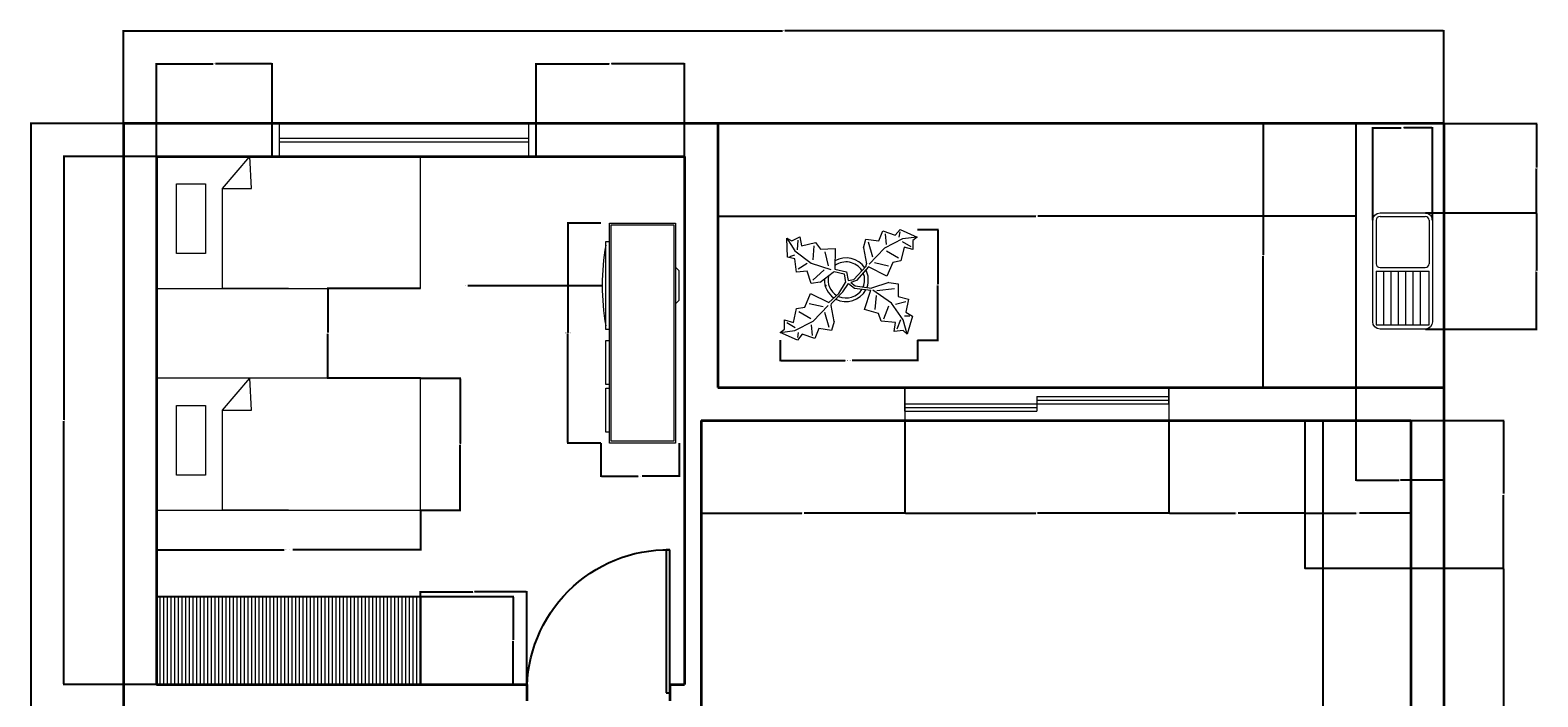
# Model space of a CAD drawing. Units: inches. Extents: x -1 to 436, y -13 to 497.
# Tile 4 of 4: x -1 to 410, y 315 to 497. Entities that reach past the tile are written whole.
import ezdxf

# ---------------------------------------------------------------- set-up
doc = ezdxf.new("R2010")
doc.units = ezdxf.units.IN
for name, color, linetype, lineweight in [('A-ANNO-DIMS', 2, 'Continuous', 18), ('A-DOOR', 4, 'Continuous', 25), ('A-FLOR-CASE', 8, 'Continuous', 25), ('A-FLOR-CASE-PATT', 9, 'Continuous', 13), ('A-FLOR-FIXT', 9, 'Continuous', 18), ('A-FURN', 8, 'Continuous', 18), ('A-GLAZ', 4, 'Continuous', 18), ('A-PLNT', 3, 'Continuous', 13), ('A-WALL', 7, 'Continuous', 35)]:
    doc.layers.add(name, color=color, linetype=linetype, lineweight=lineweight)
doc.styles.get("Standard").update_dxf_attribs({"font": 'arial.ttf'})
doc.dimstyles.get("Standard").update_dxf_attribs({"dimtxt": 0.18, "dimasz": 0.18, "dimexe": 0.18, "dimexo": 0.0625, "dimgap": 0.09, "dimtad": 0, "dimtih": 1, "dimtoh": 1, "dimdec": 4, "dimzin": 0, "dimdsep": 46, "dimtxsty": 'Standard', "dimcen": 0.09, "dimadec": 0, "dimazin": 0, "dimtfac": 1, "dimtdec": 4, "dimtofl": 0, "dimtmove": 0, "dimatfit": 3, "dimfxl": 1, "dimtolj": 1, "dimtzin": 0, "dimarcsym": 0})

# ---------------------------------------------------------------- blocks, each defined once
blk = doc.blocks.new('Plant - Rubber or Philodendron')
for p, q in [((8.8871, 10.7908), (9.9809, 13.4933)), ((9.9809, 13.4933), (13.3837, 12.301)), ((10.5828, 12.6946), (10.8893, 9.7953)), ((13.3837, 12.301), (14.68, 13.9039)), ((14.5816, 13.2037), (14.3848, 11.8033)), ((14.68, 13.9039), (19.3848, 11.8146)), ((-16.2005, 11.4774), (-13.9899, 8.1064)), ((-16.2005, 11.4774), (-14.8639, 10.7964)), ((-16.0159, 6.3329), (-16.2005, 11.4774)), ((-14.8639, 10.7964), (-12.6195, 11.8975)), ((-13.3174, 8.325), (-13.0735, 11.0065)), ((-12.6195, 11.8975), (-12.1909, 9.4345)), ((-12.1909, 9.4345), (-8.3829, 10.3)), ((-8.8369, 9.409), (-9.0894, 5.6095)), ((-8.3829, 10.3), (-7.0549, 8.501)), ((-7.0549, 8.501), (-3.0284, 8.6941)), ((-3.0284, 8.6941), (-3.0709, 3.1041)), ((4.6914, 8.8812), (5.3859, 11.2828)), ((4.6914, 8.8812), (5.5014, 4.4831)), ((5.3859, 11.2828), (8.8871, 10.7908)), ((5.9878, 10.4842), (7.1971, 6.3869)), ((10.3916, 8.7942), (6.2847, 4.4028)), ((15.3859, 11.3055), (10.3916, 8.7942)), ((15.7909, 9.1065), (14.8995, 5.3044)), ((15.2875, 10.6053), (17.5907, 9.2105)), ((19.3848, 11.8146), (15.3859, 11.3055)), ((18.1925, 8.4119), (15.7909, 9.1065)), ((19.3848, 11.8146), (18.1868, 10.9119)), ((18.1868, 10.9119), (18.1925, 8.4119)), ((-14.0069, 5.8704), (-16.0159, 6.3329)), ((-15.3434, 6.5514), (-13.9984, 6.9884)), ((-13.5868, 2.2894), (-14.0069, 5.8704)), ((-13.9899, 8.1064), (-9.5434, 4.7185)), ((-13.1329, 3.1804), (-10.6614, 4.727)), ((-9.5434, 4.7185), (-4.1917, 2.9888)), ((-4.8529, 4.012), (-5.7184, 7.82)), ((5.4346, 3.9146), (5.5014, 4.4831)), ((7.7005, 4.8881), (11.5025, 3.9967)), ((14.2977, 6.1031), (10.9934, 7.9956)), ((12.7005, 4.8994), (11.1089, 1.1958)), ((14.8995, 5.3044), (12.7005, 4.8994)), ((-10.6784, 2.491), (-13.5868, 2.2894)), ((-9.5858, -0.8715), (-10.6784, 2.491)), ((-9.1318, 0.0195), (-5.9793, 2.9025)), ((-7.1228, -0.443), (-3.5248, 2.2131)), ((-3.5248, 2.2131), (-3.3011, 2.4355)), ((-3.3011, 2.4355), (-0.5306, 1.7947)), ((-3.0709, 3.1041), (0.0797, 2.3163)), ((-0.5306, 1.7947), (-0.2255, -0.5527)), ((-0.5306, 1.7947), (-0.5306, 1.7947)), ((0.0797, 2.3163), (0.4866, -0.031)), ((0.4866, -0.031), (2.1141, 0.2298)), ((2.1141, 0.2298), (5.4346, 3.9146)), ((6.1032, 3.6844), (2.8262, -0.031)), ((11.1089, 1.1958), (6.1032, 3.6844)), ((-11.3237, -7.2629), (-9.7321, -3.5593)), ((-9.7321, -3.5593), (-4.7264, -6.0479)), ((-7.1228, -0.443), (-9.5858, -0.8715)), ((-2.019, -3.6148), (-4.7264, -6.0479)), ((-4.0579, -6.2781), (-0.9375, -3.1608)), ((-2.019, -3.6148), (-0.2255, -0.5527)), ((-0.9375, -3.1608), (0.5883, -0.8135)), ((0.5883, -0.8135), (2.2447, -2.0916)), ((2.8262, -0.031), (1.3003, -0.5527)), ((1.3003, -0.5527), (2.4193, -1.4655)), ((2.2447, -2.0916), (6.7108, -2.6626)), ((2.4193, -1.4655), (6.895, -2.1175)), ((4.943, -7.9659), (6.7108, -2.6626)), ((11.6605, -0.5413), (6.895, -2.1175)), ((12.3677, -6.1981), (7.219, -2.6772)), ((8.125, -4.0768), (7.7715, -7.9659)), ((8.3544, -2.7453), (13.1973, -2.1704)), ((11.6605, -0.5413), (14.1354, -0.8948)), ((14.1354, -0.8948), (14.1354, -4.4304)), ((-14.4141, -11.4699), (-13.5228, -7.6679)), ((-13.5228, -7.6679), (-11.3237, -7.2629)), ((-6.3237, -7.2516), (-10.1257, -6.3602)), ((-9.0148, -11.1577), (-4.9047, -6.8122)), ((-4.1246, -6.8466), (-4.0579, -6.2781)), ((-3.3146, -11.2447), (-4.1246, -6.8466)), ((8.8321, -9.0266), (4.943, -7.9659)), ((10.2463, -10.4408), (11.6605, -6.9053)), ((15.5496, -10.7943), (12.3677, -6.1981)), ((16.2567, -5.8446), (13.4283, -6.5517)), ((14.1354, -4.4304), (16.9638, -5.1375)), ((16.9638, -5.1375), (16.2567, -8.673)), ((-16.8157, -10.7754), (-14.4141, -11.4699)), ((-16.8101, -13.2754), (-16.8157, -10.7754)), ((-13.9107, -12.9688), (-16.2139, -11.574)), ((-14.0091, -13.669), (-9.0148, -11.1577)), ((-12.921, -8.4665), (-9.6166, -10.359)), ((-9.206, -15.0581), (-9.5126, -12.1588)), ((-4.611, -12.8477), (-5.8203, -8.7504)), ((-3.3146, -11.2447), (-4.0092, -13.6463)), ((9.5392, -11.1479), (8.8321, -9.0266)), ((13.4283, -11.5015), (9.5392, -11.1479)), ((13.0748, -13.9763), (13.4283, -11.5015)), ((14.8425, -10.7943), (13.7819, -13.2692)), ((16.6103, -14.6834), (15.5496, -10.7943)), ((17.3174, -9.7337), (15.9032, -9.7337)), ((16.2567, -8.673), (18.0245, -9.7337)), ((18.0245, -9.7337), (16.6103, -14.6834)), ((-18.008, -14.1781), (-16.8101, -13.2754)), ((-18.008, -14.1781), (-14.0091, -13.669)), ((-13.3032, -16.2674), (-18.008, -14.1781)), ((-12.0069, -14.6645), (-13.3032, -16.2674)), ((-13.2048, -15.5672), (-13.008, -14.1668)), ((-8.6042, -15.8568), (-12.0069, -14.6645)), ((-7.5103, -13.1543), (-8.6042, -15.8568)), ((-4.0092, -13.6463), (-7.5103, -13.1543)), ((15.5496, -13.6228), (13.0748, -13.9763)), ((16.6103, -14.6834), (15.5496, -13.6228))]:
    blk.add_line(p, q)
for centre, radius, start, end in [((0, 0), 6.1275, 34.37569, 120.1028), ((-0.0601, -0.2075), 5.2461, 33.82192, 124.9414), ((0.0308, 0.1664), 6, 178.6147, 235.1169), ((0.0308, 0.1664), 5, 168.1647, 238.6725), ((-0.2664, 0.1682), 5.2775, 338.4094, 20.03007), ((-0.098, 0.1364), 6.1288, 341.2017, 26.09184), ((-0.0234, 0.3825), 6.1492, 242.5812, 331.2714), ((-0.1102, 0.4886), 5.2883, 247.3711, 327.472)]:
    blk.add_arc(centre, radius, start, end)
blk = doc.blocks.new('Entertainment Center')
for p, q in [((-4, 0), (-5, -1)), ((4, 0), (-4, 0)), ((5, -1), (4, 0)), ((-17, -19), (-17, -1)), ((-17, -1), (43, -1)), ((-16.5, -18.5), (-16.5, -1.5)), ((-16.5, -1.5), (42.5, -1.5)), ((42.5, -1.5), (42.5, -18.5)), ((43, -1), (43, -19)), ((43, -19), (-17, -19)), ((42.5, -18.5), (-16.5, -18.5)), ((-12, -20), (-12, -19)), ((12, -20), (-12, -20)), ((12, -19), (12, -20)), ((15, -20), (15, -19)), ((27, -20), (15, -20)), ((27, -19), (27, -20)), ((28, -20), (28, -19)), ((40, -20), (28, -20)), ((40, -19), (40, -20))]:
    blk.add_line(p, q)
blk.add_arc((0, 40), 61, 259.6111, 280.3889)
blk = doc.blocks.new('BED-TWIN-36X72')
for p, q in [((72, 36), (0, 36)), ((0, 36), (0, 0)), ((18, 27.25), (25.41, 36)), ((25.93, 27.25), (25.41, 36)), ((72, 0), (72, 36)), ((18, 0), (18, 27.25)), ((18, 27.25), (25.93, 27.25)), ((0, 0), (72, 0)), ((24, 0), (18, 0)), ((36, 0), (24, 0))]:
    blk.add_line(p, q)
blk.add_lwpolyline([(5.46, 28.55), (13.32, 28.55), (13.32, 9.55), (5.46, 9.55)], close=True)
blk = doc.blocks.new('DOOR-SGL-39')
for p, q in [((38, 0), (38, 39)), ((38, 39), (39, 39)), ((39, 39), (39, 0)), ((39, 0), (38, 0))]:
    blk.add_line(p, q)
blk.add_arc((38.5, 38.5), 38.5, 179.2559, 270.7441)
blk = doc.blocks.new('WIN-FIXED-72')
for p, q in [((2, 0), (2, 9)), ((70, 0), (70, 9)), ((2, 5), (70, 5)), ((2, 4), (70, 4))]:
    blk.add_line(p, q)
blk.add_lwpolyline([(0, 9), (72, 9), (72, 0), (0, 0)], close=True)
blk = doc.blocks.new('*D12')
at = {"layer": 'A-ANNO-DIMS', "color": 0, "lineweight": -2, "transparency": 16777216}
for p, q in [((33, 366.03), (33, 355.11)), ((105, 366.03), (105, 355.11)), ((33.18, 355.29), (67.82, 355.29)), ((104.82, 355.29), (70.18, 355.29))]:
    blk.add_line(p, q, dxfattribs=at)
at = {"layer": 'A-ANNO-DIMS', "color": 0, "transparency": 16777216}
for points in [[(33.18, 355.32), (33.18, 355.26), (33, 355.29)], [(104.82, 355.32), (104.82, 355.26), (105, 355.29)]]:
    blk.add_solid(points, dxfattribs=at)
at = {"layer": 'Defpoints', "color": 0, "transparency": 16777216}
for p in [(33, 366.09), (105, 366.09), (105, 355.29)]:
    blk.add_point(p, dxfattribs=at)
at = {"layer": 'A-ANNO-DIMS', "color": 0, "transparency": 16777216, "insert": (69, 355.29), "char_height": 0.18, "attachment_point": 5}
blk.add_mtext('\\A1;TWIN BED 72 TYP.', dxfattribs=at)
blk = doc.blocks.new('*D13')
at = {"layer": 'A-ANNO-DIMS', "color": 0, "lineweight": -2, "transparency": 16777216}
for p, q in [((105.06, 402.09), (115.98, 402.09)), ((115.8, 401.91), (115.8, 384.27)), ((115.8, 366.27), (115.8, 383.91)), ((105.06, 366.09), (115.98, 366.09))]:
    blk.add_line(p, q, dxfattribs=at)
at = {"layer": 'A-ANNO-DIMS', "color": 0, "transparency": 16777216}
for points in [[(115.77, 401.91), (115.83, 401.91), (115.8, 402.09)], [(115.77, 366.27), (115.83, 366.27), (115.8, 366.09)]]:
    blk.add_solid(points, dxfattribs=at)
at = {"layer": 'Defpoints', "color": 0, "transparency": 16777216}
for p in [(105, 402.09), (115.8, 402.09), (105, 366.09)]:
    blk.add_point(p, dxfattribs=at)
at = {"layer": 'A-ANNO-DIMS', "color": 0, "transparency": 16777216, "insert": (115.8, 384.09), "char_height": 0.18, "attachment_point": 5}
blk.add_mtext('\\A1;36 TYP.', dxfattribs=at)
blk = doc.blocks.new('*D16')
at = {"layer": 'A-ANNO-DIMS', "color": 0, "lineweight": -2, "transparency": 16777216}
for p, q in [((154.11, 444.37), (144.99, 444.37)), ((145.17, 444.19), (145.17, 414.55)), ((145.17, 384.55), (145.17, 414.18)), ((154.11, 384.37), (144.99, 384.37))]:
    blk.add_line(p, q, dxfattribs=at)
at = {"layer": 'A-ANNO-DIMS', "color": 0, "transparency": 16777216}
for points in [[(145.14, 444.19), (145.2, 444.19), (145.17, 444.37)], [(145.14, 384.55), (145.2, 384.55), (145.17, 384.37)]]:
    blk.add_solid(points, dxfattribs=at)
at = {"layer": 'Defpoints', "color": 0, "transparency": 16777216}
for p in [(154.17, 444.37), (145.17, 384.37), (154.17, 384.37)]:
    blk.add_point(p, dxfattribs=at)
at = {"layer": 'A-ANNO-DIMS', "color": 0, "transparency": 16777216, "insert": (145.17, 414.37), "char_height": 0.18, "attachment_point": 5}
blk.add_mtext('\\A1;MEDIA UNIT 60 TYP.', dxfattribs=at)
blk = doc.blocks.new('*D17')
at = {"layer": 'A-ANNO-DIMS', "color": 0, "lineweight": -2, "transparency": 16777216}
for p, q in [((154.17, 384.3), (154.17, 375.19)), ((175.5, 384.3), (175.5, 375.19)), ((154.35, 375.37), (164.31, 375.37)), ((175.32, 375.37), (165.37, 375.37))]:
    blk.add_line(p, q, dxfattribs=at)
at = {"layer": 'A-ANNO-DIMS', "color": 0, "transparency": 16777216}
for points in [[(154.35, 375.4), (154.35, 375.34), (154.17, 375.37)], [(175.32, 375.4), (175.32, 375.34), (175.5, 375.37)]]:
    blk.add_solid(points, dxfattribs=at)
at = {"layer": 'Defpoints', "color": 0, "transparency": 16777216}
for p in [(154.17, 384.37), (175.5, 384.37), (175.5, 375.37)]:
    blk.add_point(p, dxfattribs=at)
at = {"layer": 'A-ANNO-DIMS', "color": 0, "transparency": 16777216, "insert": (164.84, 375.37), "char_height": 0.18, "attachment_point": 5}
blk.add_mtext('\\A1;21 TYP.', dxfattribs=at)
blk = doc.blocks.new('*D26')
at = {"layer": 'A-ANNO-DIMS', "color": 0, "lineweight": -2, "transparency": 16777216}
for p, q in [((203.04, 412.39), (203.04, 406.66)), ((240.44, 412.39), (240.44, 406.66)), ((203.22, 406.84), (220.78, 406.84)), ((240.26, 406.84), (222.7, 406.84))]:
    blk.add_line(p, q, dxfattribs=at)
at = {"layer": 'A-ANNO-DIMS', "color": 0, "transparency": 16777216}
for points in [[(203.22, 406.87), (203.22, 406.81), (203.04, 406.84)], [(240.26, 406.87), (240.26, 406.81), (240.44, 406.84)]]:
    blk.add_solid(points, dxfattribs=at)
at = {"layer": 'Defpoints', "color": 0, "transparency": 16777216}
for p in [(203.04, 412.45), (240.44, 412.45), (240.44, 406.84)]:
    blk.add_point(p, dxfattribs=at)
at = {"layer": 'A-ANNO-DIMS', "color": 0, "transparency": 16777216, "insert": (221.74, 406.84), "char_height": 0.18, "attachment_point": 5}
blk.add_mtext('\\A1;PLANT 37 TYP.', dxfattribs=at)
blk = doc.blocks.new('*D27')
at = {"layer": 'A-ANNO-DIMS', "color": 0, "lineweight": -2, "transparency": 16777216}
for p, q in [((240.5, 442.62), (246.23, 442.62)), ((246.05, 442.44), (246.05, 427.72)), ((246.05, 412.63), (246.05, 427.36)), ((240.5, 412.45), (246.23, 412.45))]:
    blk.add_line(p, q, dxfattribs=at)
at = {"layer": 'A-ANNO-DIMS', "color": 0, "transparency": 16777216}
for points in [[(246.02, 442.44), (246.08, 442.44), (246.05, 442.62)], [(246.02, 412.63), (246.08, 412.63), (246.05, 412.45)]]:
    blk.add_solid(points, dxfattribs=at)
at = {"layer": 'Defpoints', "color": 0, "transparency": 16777216}
for p in [(240.44, 442.62), (246.05, 442.62), (240.44, 412.45)]:
    blk.add_point(p, dxfattribs=at)
at = {"layer": 'A-ANNO-DIMS', "color": 0, "transparency": 16777216, "insert": (246.05, 427.54), "char_height": 0.18, "attachment_point": 5}
blk.add_mtext('\\A1;30 TYP.', dxfattribs=at)
blk = doc.blocks.new('*D28')
at = {"layer": 'A-ANNO-DIMS', "color": 0, "lineweight": -2, "transparency": 16777216}
for p, q in [((24, 471.6), (24, 496.96)), ((24.18, 496.78), (203.71, 496.78)), ((383.82, 496.78), (204.29, 496.78)), ((384, 471.6), (384, 496.96))]:
    blk.add_line(p, q, dxfattribs=at)
at = {"layer": 'A-ANNO-DIMS', "color": 0, "transparency": 16777216}
for points in [[(24.18, 496.81), (24.18, 496.75), (24, 496.78)], [(383.82, 496.81), (383.82, 496.75), (384, 496.78)]]:
    blk.add_solid(points, dxfattribs=at)
at = {"layer": 'Defpoints', "color": 0, "transparency": 16777216}
for p in [(384, 496.78), (24, 471.53), (384, 471.53)]:
    blk.add_point(p, dxfattribs=at)
at = {"layer": 'A-ANNO-DIMS', "color": 0, "transparency": 16777216, "insert": (204, 496.78), "char_height": 0.18, "attachment_point": 5}
blk.add_mtext('\\A1;360', dxfattribs=at)
blk = doc.blocks.new('*D29')
at = {"layer": 'A-ANNO-DIMS', "color": 0, "lineweight": -2, "transparency": 16777216}
for p, q in [((23.94, 471.53), (-1.43, 471.53)), ((-1.25, 471.35), (-1.25, 242.22)), ((-1.25, 12.71), (-1.25, 241.85)), ((23.94, 12.53), (-1.43, 12.53))]:
    blk.add_line(p, q, dxfattribs=at)
at = {"layer": 'A-ANNO-DIMS', "color": 0, "transparency": 16777216}
for points in [[(-1.28, 471.35), (-1.22, 471.35), (-1.25, 471.53)], [(-1.28, 12.71), (-1.22, 12.71), (-1.25, 12.53)]]:
    blk.add_solid(points, dxfattribs=at)
at = {"layer": 'Defpoints', "color": 0, "transparency": 16777216}
for p in [(-1.25, 471.53), (24, 471.53), (24, 12.53)]:
    blk.add_point(p, dxfattribs=at)
at = {"layer": 'A-ANNO-DIMS', "color": 0, "transparency": 16777216, "insert": (-1.25, 242.03), "char_height": 0.18, "attachment_point": 5}
blk.add_mtext('\\A1;459', dxfattribs=at)
blk = doc.blocks.new('*D32')
at = {"layer": 'A-ANNO-DIMS', "color": 0, "lineweight": -2, "transparency": 16777216}
for p, q in [((33, 462.6), (33, 487.96)), ((33.18, 487.78), (48.43, 487.78)), ((64.32, 487.78), (49.07, 487.78)), ((64.5, 462.6), (64.5, 487.96))]:
    blk.add_line(p, q, dxfattribs=at)
at = {"layer": 'A-ANNO-DIMS', "color": 0, "transparency": 16777216}
for points in [[(33.18, 487.81), (33.18, 487.75), (33, 487.78)], [(64.32, 487.81), (64.32, 487.75), (64.5, 487.78)]]:
    blk.add_solid(points, dxfattribs=at)
at = {"layer": 'Defpoints', "color": 0, "transparency": 16777216}
for p in [(64.5, 487.78), (33, 462.53), (64.5, 462.53)]:
    blk.add_point(p, dxfattribs=at)
at = {"layer": 'A-ANNO-DIMS', "color": 0, "transparency": 16777216, "insert": (48.75, 487.78), "char_height": 0.18, "attachment_point": 5}
blk.add_mtext('\\A1;31.5', dxfattribs=at)
blk = doc.blocks.new('*D33')
at = {"layer": 'A-ANNO-DIMS', "color": 0, "lineweight": -2, "transparency": 16777216}
for p, q in [((136.5, 462.6), (136.5, 487.96)), ((136.68, 487.78), (156.42, 487.78)), ((176.82, 487.78), (157.08, 487.78)), ((177, 462.6), (177, 487.96))]:
    blk.add_line(p, q, dxfattribs=at)
at = {"layer": 'A-ANNO-DIMS', "color": 0, "transparency": 16777216}
for points in [[(136.68, 487.81), (136.68, 487.75), (136.5, 487.78)], [(176.82, 487.81), (176.82, 487.75), (177, 487.78)]]:
    blk.add_solid(points, dxfattribs=at)
at = {"layer": 'Defpoints', "color": 0, "transparency": 16777216}
for p in [(177, 487.78), (136.5, 462.53), (177, 462.53)]:
    blk.add_point(p, dxfattribs=at)
at = {"layer": 'A-ANNO-DIMS', "color": 0, "transparency": 16777216, "insert": (156.75, 487.78), "char_height": 0.18, "attachment_point": 5}
blk.add_mtext('\\A1;40.5', dxfattribs=at)
blk = doc.blocks.new('*D34')
at = {"layer": 'A-ANNO-DIMS', "color": 0, "lineweight": -2, "transparency": 16777216}
for p, q in [((186, 471.47), (186, 446.1)), ((360, 471.47), (360, 446.1)), ((186.18, 446.28), (272.72, 446.28)), ((359.82, 446.28), (273.28, 446.28))]:
    blk.add_line(p, q, dxfattribs=at)
at = {"layer": 'A-ANNO-DIMS', "color": 0, "transparency": 16777216}
for points in [[(186.18, 446.31), (186.18, 446.25), (186, 446.28)], [(359.82, 446.31), (359.82, 446.25), (360, 446.28)]]:
    blk.add_solid(points, dxfattribs=at)
at = {"layer": 'Defpoints', "color": 0, "transparency": 16777216}
for p in [(186, 471.53), (360, 471.53), (186, 446.28)]:
    blk.add_point(p, dxfattribs=at)
at = {"layer": 'A-ANNO-DIMS', "color": 0, "transparency": 16777216, "insert": (273, 446.28), "char_height": 0.18, "attachment_point": 5}
blk.add_mtext('\\A1;174', dxfattribs=at)
blk = doc.blocks.new('*D35')
at = {"layer": 'A-ANNO-DIMS', "color": 0, "lineweight": -2, "transparency": 16777216}
for p, q in [((360, 399.47), (360, 374.1)), ((384, 399.47), (384, 374.1)), ((360.18, 374.28), (371.78, 374.28)), ((383.82, 374.28), (372.22, 374.28))]:
    blk.add_line(p, q, dxfattribs=at)
at = {"layer": 'A-ANNO-DIMS', "color": 0, "transparency": 16777216}
for points in [[(360.18, 374.31), (360.18, 374.25), (360, 374.28)], [(383.82, 374.31), (383.82, 374.25), (384, 374.28)]]:
    blk.add_solid(points, dxfattribs=at)
at = {"layer": 'Defpoints', "color": 0, "transparency": 16777216}
for p in [(360, 399.53), (384, 399.53), (360, 374.28)]:
    blk.add_point(p, dxfattribs=at)
at = {"layer": 'A-ANNO-DIMS', "color": 0, "transparency": 16777216, "insert": (372, 374.28), "char_height": 0.18, "attachment_point": 5}
blk.add_mtext('\\A1;24', dxfattribs=at)
blk = doc.blocks.new('*D36')
at = {"layer": 'A-ANNO-DIMS', "color": 0, "lineweight": -2, "transparency": 16777216}
for p, q in [((181.5, 390.47), (181.5, 365.1)), ((237, 390.47), (237, 365.1)), ((181.68, 365.28), (208.93, 365.28)), ((236.82, 365.28), (209.57, 365.28))]:
    blk.add_line(p, q, dxfattribs=at)
at = {"layer": 'A-ANNO-DIMS', "color": 0, "transparency": 16777216}
for points in [[(181.68, 365.31), (181.68, 365.25), (181.5, 365.28)], [(236.82, 365.31), (236.82, 365.25), (237, 365.28)]]:
    blk.add_solid(points, dxfattribs=at)
at = {"layer": 'Defpoints', "color": 0, "transparency": 16777216}
for p in [(181.5, 390.53), (237, 390.53), (181.5, 365.28)]:
    blk.add_point(p, dxfattribs=at)
at = {"layer": 'A-ANNO-DIMS', "color": 0, "transparency": 16777216, "insert": (209.25, 365.28), "char_height": 0.18, "attachment_point": 5}
blk.add_mtext('\\A1;55.5', dxfattribs=at)
blk = doc.blocks.new('*D37')
at = {"layer": 'A-ANNO-DIMS', "color": 0, "lineweight": -2, "transparency": 16777216}
for p, q in [((237, 390.47), (237, 365.1)), ((309, 390.47), (309, 365.1)), ((237.18, 365.28), (272.78, 365.28)), ((308.82, 365.28), (273.22, 365.28))]:
    blk.add_line(p, q, dxfattribs=at)
at = {"layer": 'A-ANNO-DIMS', "color": 0, "transparency": 16777216}
for points in [[(237.18, 365.31), (237.18, 365.25), (237, 365.28)], [(308.82, 365.31), (308.82, 365.25), (309, 365.28)]]:
    blk.add_solid(points, dxfattribs=at)
at = {"layer": 'Defpoints', "color": 0, "transparency": 16777216}
for p in [(237, 390.53), (309, 390.53), (237, 365.28)]:
    blk.add_point(p, dxfattribs=at)
at = {"layer": 'A-ANNO-DIMS', "color": 0, "transparency": 16777216, "insert": (273, 365.28), "char_height": 0.18, "attachment_point": 5}
blk.add_mtext('\\A1;72', dxfattribs=at)
blk = doc.blocks.new('*D38')
at = {"layer": 'A-ANNO-DIMS', "color": 0, "lineweight": -2, "transparency": 16777216}
for p, q in [((309, 390.47), (309, 365.1)), ((346.13, 390.47), (346.13, 365.1)), ((309.18, 365.28), (327.17, 365.28)), ((345.95, 365.28), (327.96, 365.28))]:
    blk.add_line(p, q, dxfattribs=at)
at = {"layer": 'A-ANNO-DIMS', "color": 0, "transparency": 16777216}
for points in [[(309.18, 365.31), (309.18, 365.25), (309, 365.28)], [(345.95, 365.31), (345.95, 365.25), (346.13, 365.28)]]:
    blk.add_solid(points, dxfattribs=at)
at = {"layer": 'Defpoints', "color": 0, "transparency": 16777216}
for p in [(309, 390.53), (346.13, 390.53), (309, 365.28)]:
    blk.add_point(p, dxfattribs=at)
at = {"layer": 'A-ANNO-DIMS', "color": 0, "transparency": 16777216, "insert": (327.57, 365.28), "char_height": 0.18, "attachment_point": 5}
blk.add_mtext('\\A1;37.13', dxfattribs=at)
blk = doc.blocks.new('*D39')
at = {"layer": 'A-ANNO-DIMS', "color": 0, "lineweight": -2, "transparency": 16777216}
for p, q in [((346.13, 390.47), (346.13, 365.1)), ((375, 390.47), (375, 365.1)), ((346.31, 365.28), (360.1, 365.28)), ((374.82, 365.28), (361.03, 365.28))]:
    blk.add_line(p, q, dxfattribs=at)
at = {"layer": 'A-ANNO-DIMS', "color": 0, "transparency": 16777216}
for points in [[(346.31, 365.31), (346.31, 365.25), (346.13, 365.28)], [(374.82, 365.31), (374.82, 365.25), (375, 365.28)]]:
    blk.add_solid(points, dxfattribs=at)
at = {"layer": 'Defpoints', "color": 0, "transparency": 16777216}
for p in [(346.13, 390.53), (375, 390.53), (346.13, 365.28)]:
    blk.add_point(p, dxfattribs=at)
at = {"layer": 'A-ANNO-DIMS', "color": 0, "transparency": 16777216, "insert": (360.57, 365.28), "char_height": 0.18, "attachment_point": 5}
blk.add_mtext('\\A1;28.866', dxfattribs=at)
blk = doc.blocks.new('*D40')
at = {"layer": 'A-ANNO-DIMS', "color": 0, "lineweight": -2, "transparency": 16777216}
for p, q in [((359.94, 471.53), (334.57, 471.53)), ((334.75, 471.35), (334.75, 435.71)), ((334.75, 399.71), (334.75, 435.35)), ((359.94, 399.53), (334.57, 399.53))]:
    blk.add_line(p, q, dxfattribs=at)
at = {"layer": 'A-ANNO-DIMS', "color": 0, "transparency": 16777216}
for points in [[(334.72, 471.35), (334.78, 471.35), (334.75, 471.53)], [(334.72, 399.71), (334.78, 399.71), (334.75, 399.53)]]:
    blk.add_solid(points, dxfattribs=at)
at = {"layer": 'Defpoints', "color": 0, "transparency": 16777216}
for p in [(334.75, 471.53), (360, 471.53), (360, 399.53)]:
    blk.add_point(p, dxfattribs=at)
at = {"layer": 'A-ANNO-DIMS', "color": 0, "transparency": 16777216, "insert": (334.75, 435.53), "char_height": 0.18, "attachment_point": 5}
blk.add_mtext('\\A1;72', dxfattribs=at)
blk = doc.blocks.new('*D41')
at = {"layer": 'A-ANNO-DIMS', "color": 0, "lineweight": -2, "transparency": 16777216}
for p, q in [((375.06, 390.53), (400.43, 390.53)), ((400.25, 390.35), (400.25, 370.57)), ((400.25, 350.42), (400.25, 370.2)), ((375.06, 350.24), (400.43, 350.24))]:
    blk.add_line(p, q, dxfattribs=at)
at = {"layer": 'A-ANNO-DIMS', "color": 0, "transparency": 16777216}
for points in [[(400.22, 390.35), (400.28, 390.35), (400.25, 390.53)], [(400.22, 350.42), (400.28, 350.42), (400.25, 350.24)]]:
    blk.add_solid(points, dxfattribs=at)
at = {"layer": 'Defpoints', "color": 0, "transparency": 16777216}
for p in [(375, 390.53), (375, 350.24), (400.25, 350.24)]:
    blk.add_point(p, dxfattribs=at)
at = {"layer": 'A-ANNO-DIMS', "color": 0, "transparency": 16777216, "insert": (400.25, 370.39), "char_height": 0.18, "attachment_point": 5}
blk.add_mtext('\\A1;40.295', dxfattribs=at)
blk = doc.blocks.new('*D42')
at = {"layer": 'A-ANNO-DIMS', "color": 0, "lineweight": -2, "transparency": 16777216}
for p, q in [((375.06, 350.24), (400.43, 350.24)), ((400.25, 350.06), (400.25, 306.27)), ((400.25, 262.12), (400.25, 305.91)), ((375.06, 261.94), (400.43, 261.94))]:
    blk.add_line(p, q, dxfattribs=at)
at = {"layer": 'A-ANNO-DIMS', "color": 0, "transparency": 16777216}
for points in [[(400.22, 350.06), (400.28, 350.06), (400.25, 350.24)], [(400.22, 262.12), (400.28, 262.12), (400.25, 261.94)]]:
    blk.add_solid(points, dxfattribs=at)
at = {"layer": 'Defpoints', "color": 0, "transparency": 16777216}
for p in [(375, 350.24), (375, 261.94), (400.25, 261.94)]:
    blk.add_point(p, dxfattribs=at)
at = {"layer": 'A-ANNO-DIMS', "color": 0, "transparency": 16777216, "insert": (400.25, 306.09), "char_height": 0.18, "attachment_point": 5}
blk.add_mtext('\\A1;88.3', dxfattribs=at)
blk = doc.blocks.new('*D49')
at = {"layer": 'A-ANNO-DIMS', "color": 0, "lineweight": -2, "transparency": 16777216}
for p, q in [((32.94, 462.53), (7.57, 462.53)), ((7.75, 462.35), (7.75, 390.71)), ((7.75, 318.71), (7.75, 390.35)), ((32.94, 318.53), (7.57, 318.53))]:
    blk.add_line(p, q, dxfattribs=at)
at = {"layer": 'A-ANNO-DIMS', "color": 0, "transparency": 16777216}
for points in [[(7.72, 462.35), (7.78, 462.35), (7.75, 462.53)], [(7.72, 318.71), (7.78, 318.71), (7.75, 318.53)]]:
    blk.add_solid(points, dxfattribs=at)
at = {"layer": 'Defpoints', "color": 0, "transparency": 16777216}
for p in [(7.75, 462.53), (33, 462.53), (33, 318.53)]:
    blk.add_point(p, dxfattribs=at)
at = {"layer": 'A-ANNO-DIMS', "color": 0, "transparency": 16777216, "insert": (7.75, 390.53), "char_height": 0.18, "attachment_point": 5}
blk.add_mtext('\\A1;144', dxfattribs=at)
blk = doc.blocks.new('*D62')
at = {"layer": 'A-ANNO-DIMS', "color": 0, "lineweight": -2, "transparency": 16777216}
for p, q in [((104.94, 426.53), (79.57, 426.53)), ((79.75, 426.35), (79.75, 414.49)), ((79.75, 402.27), (79.75, 414.13)), ((104.94, 402.09), (79.57, 402.09))]:
    blk.add_line(p, q, dxfattribs=at)
at = {"layer": 'A-ANNO-DIMS', "color": 0, "transparency": 16777216}
for points in [[(79.72, 426.35), (79.78, 426.35), (79.75, 426.53)], [(79.72, 402.27), (79.78, 402.27), (79.75, 402.09)]]:
    blk.add_solid(points, dxfattribs=at)
at = {"layer": 'Defpoints', "color": 0, "transparency": 16777216}
for p in [(79.75, 426.53), (105, 426.53), (105, 402.09)]:
    blk.add_point(p, dxfattribs=at)
at = {"layer": 'A-ANNO-DIMS', "color": 0, "transparency": 16777216, "insert": (79.75, 414.31), "char_height": 0.18, "attachment_point": 5}
blk.add_mtext('\\A1;24.44', dxfattribs=at)
blk = doc.blocks.new('*D63')
at = {"layer": 'A-ANNO-DIMS', "color": 0, "lineweight": -2, "transparency": 16777216}
for p, q in [((105.06, 342.53), (130.43, 342.53)), ((130.25, 342.35), (130.25, 330.71)), ((130.25, 318.71), (130.25, 330.35)), ((105.06, 318.53), (130.43, 318.53))]:
    blk.add_line(p, q, dxfattribs=at)
at = {"layer": 'A-ANNO-DIMS', "color": 0, "transparency": 16777216}
for points in [[(130.22, 342.35), (130.28, 342.35), (130.25, 342.53)], [(130.22, 318.71), (130.28, 318.71), (130.25, 318.53)]]:
    blk.add_solid(points, dxfattribs=at)
at = {"layer": 'Defpoints', "color": 0, "transparency": 16777216}
for p in [(105, 342.53), (105, 318.53), (130.25, 318.53)]:
    blk.add_point(p, dxfattribs=at)
at = {"layer": 'A-ANNO-DIMS', "color": 0, "transparency": 16777216, "insert": (130.25, 330.53), "char_height": 0.18, "attachment_point": 5}
blk.add_mtext('\\A1;24', dxfattribs=at)
blk = doc.blocks.new('*D64')
at = {"layer": 'A-ANNO-DIMS', "color": 0, "lineweight": -2, "transparency": 16777216}
for p, q in [((105, 318.6), (105, 343.96)), ((105.18, 343.78), (119.28, 343.78)), ((133.82, 343.78), (119.72, 343.78)), ((134, 318.6), (134, 343.96))]:
    blk.add_line(p, q, dxfattribs=at)
at = {"layer": 'A-ANNO-DIMS', "color": 0, "transparency": 16777216}
for points in [[(105.18, 343.81), (105.18, 343.75), (105, 343.78)], [(133.82, 343.81), (133.82, 343.75), (134, 343.78)]]:
    blk.add_solid(points, dxfattribs=at)
at = {"layer": 'Defpoints', "color": 0, "transparency": 16777216}
for p in [(134, 343.78), (105, 318.53), (134, 318.53)]:
    blk.add_point(p, dxfattribs=at)
at = {"layer": 'A-ANNO-DIMS', "color": 0, "transparency": 16777216, "insert": (119.5, 343.78), "char_height": 0.18, "attachment_point": 5}
blk.add_mtext('\\A1;29', dxfattribs=at)
blk = doc.blocks.new('*D73')
at = {"layer": 'A-ANNO-DIMS', "color": 0, "lineweight": -2, "transparency": 16777216}
for p, q in [((378.97, 447.11), (409.43, 447.11)), ((409.25, 446.93), (409.25, 431.46)), ((409.25, 415.63), (409.25, 431.1)), ((378.97, 415.45), (409.43, 415.45))]:
    blk.add_line(p, q, dxfattribs=at)
at = {"layer": 'A-ANNO-DIMS', "color": 0, "transparency": 16777216}
for points in [[(409.22, 446.93), (409.28, 446.93), (409.25, 447.11)], [(409.22, 415.63), (409.28, 415.63), (409.25, 415.45)]]:
    blk.add_solid(points, dxfattribs=at)
at = {"layer": 'Defpoints', "color": 0, "transparency": 16777216}
for p in [(378.9, 447.11), (409.25, 447.11), (378.9, 415.45)]:
    blk.add_point(p, dxfattribs=at)
at = {"layer": 'A-ANNO-DIMS', "color": 0, "transparency": 16777216, "insert": (409.25, 431.28), "char_height": 0.18, "attachment_point": 5}
blk.add_mtext('\\A1;31.655', dxfattribs=at)
blk = doc.blocks.new('*D74')
at = {"layer": 'A-ANNO-DIMS', "color": 0, "lineweight": -2, "transparency": 16777216}
for p, q in [((384.06, 471.53), (409.43, 471.53)), ((409.25, 471.35), (409.25, 459.5)), ((409.25, 447.29), (409.25, 459.14)), ((378.97, 447.11), (409.43, 447.11))]:
    blk.add_line(p, q, dxfattribs=at)
at = {"layer": 'A-ANNO-DIMS', "color": 0, "transparency": 16777216}
for points in [[(409.22, 471.35), (409.28, 471.35), (409.25, 471.53)], [(409.22, 447.29), (409.28, 447.29), (409.25, 447.11)]]:
    blk.add_solid(points, dxfattribs=at)
at = {"layer": 'Defpoints', "color": 0, "transparency": 16777216}
for p in [(384, 471.53), (409.25, 471.53), (378.9, 447.11)]:
    blk.add_point(p, dxfattribs=at)
at = {"layer": 'A-ANNO-DIMS', "color": 0, "transparency": 16777216, "insert": (409.25, 459.32), "char_height": 0.18, "attachment_point": 5}
blk.add_mtext('\\A1;24.427', dxfattribs=at)
blk = doc.blocks.new('*D75')
at = {"layer": 'A-ANNO-DIMS', "color": 0, "lineweight": -2, "transparency": 16777216}
for p, q in [((364.59, 445.17), (364.59, 470.54)), ((364.77, 470.36), (372.38, 470.36)), ((380.72, 470.36), (373.12, 470.36)), ((380.9, 445.17), (380.9, 470.54))]:
    blk.add_line(p, q, dxfattribs=at)
at = {"layer": 'A-ANNO-DIMS', "color": 0, "transparency": 16777216}
for points in [[(364.77, 470.39), (364.77, 470.33), (364.59, 470.36)], [(380.72, 470.39), (380.72, 470.33), (380.9, 470.36)]]:
    blk.add_solid(points, dxfattribs=at)
at = {"layer": 'Defpoints', "color": 0, "transparency": 16777216}
for p in [(380.9, 470.36), (364.59, 445.11), (380.9, 445.11)]:
    blk.add_point(p, dxfattribs=at)
at = {"layer": 'A-ANNO-DIMS', "color": 0, "transparency": 16777216, "insert": (372.75, 470.36), "char_height": 0.18, "attachment_point": 5}
blk.add_mtext('\\A1;16.31', dxfattribs=at)
blk = doc.blocks.new('*D82')
at = {"layer": 'A-ANNO-DIMS', "color": 0, "lineweight": -2, "transparency": 16777216}
for p, q in [((117.9, 427.37), (154.32, 427.37)), ((215.41, 427.37), (215.59, 427.37)), ((215.5, 427.28), (215.5, 427.46))]:
    blk.add_line(p, q, dxfattribs=at)
at = {"layer": 'A-ANNO-DIMS', "color": 0, "transparency": 16777216}
blk.add_solid([(154.32, 427.4), (154.32, 427.34), (154.5, 427.37)], dxfattribs=at)
at = {"layer": 'Defpoints', "color": 0, "transparency": 16777216}
for p in [(154.5, 427.37), (215.5, 427.37)]:
    blk.add_point(p, dxfattribs=at)
at = {"layer": 'A-ANNO-DIMS', "color": 0, "transparency": 16777216, "insert": (117.42, 427.37), "char_height": 0.18, "attachment_point": 5}
blk.add_mtext('\\A1;3X R61', dxfattribs=at)

msp = doc.modelspace()

# ---------------------------------------------------------------- hatches: boundary and pattern name
at = {"layer": 'A-FLOR-CASE-PATT'}
h = msp.add_hatch(dxfattribs=at)
h.set_pattern_fill('ANSI31', color=256, scale=0.31496, angle=45, style=0)
h.paths.add_polyline_path([(33, 318.5331), (105, 318.5331), (105, 342.5331), (33, 342.5331)])

# ---------------------------------------------------------------- linework, layer by layer
at = {"layer": 'A-FLOR-CASE'}
for p, q in [((360, 471.5331), (360, 399.5331)), ((351, 390.5331), (351, 261.9384)), ((33, 342.5331), (105, 342.5331)), ((33, 342.5331), (33, 318.5331)), ((105, 342.5331), (105, 318.5331))]:
    msp.add_line(p, q, dxfattribs=at)
msp.add_lwpolyline([(375, 390.5331), (346.1337, 390.5331), (346.1337, 350.238), (375, 350.238)], close=True, dxfattribs=at)
at = {"layer": 'A-FLOR-FIXT'}
for p, q in [((365.5301, 445.1058), (365.5301, 433.2659)), ((366.5941, 446.1698), (378.9026, 446.1698)), ((379.9666, 445.1058), (379.9666, 433.2659)), ((366.5941, 432.2019), (378.9026, 432.2019)), ((365.5301, 431.2782), (379.9666, 431.2782)), ((365.5301, 431.2782), (365.5301, 416.585)), ((367.5301, 431.2782), (367.5301, 416.585)), ((369.5301, 431.2782), (369.5301, 416.585)), ((371.5301, 431.2782), (371.5301, 416.585)), ((373.5301, 431.2782), (373.5301, 416.585)), ((375.5301, 431.2782), (375.5301, 416.585)), ((377.5301, 431.2782), (377.5301, 416.585)), ((379.9796, 416.585), (379.9666, 431.2782)), ((365.5301, 416.585), (379.9796, 416.585))]:
    msp.add_line(p, q, dxfattribs=at)
msp.add_lwpolyline([(366.5941, 447.1058), (378.9026, 447.1058, -0.41421356), (380.9026, 445.1058), (380.9026, 417.4505, -0.41421356), (378.9026, 415.4505), (366.5941, 415.4505, -0.41421356), (364.5941, 417.4505), (364.5941, 445.1058, -0.41421356)], format="xyb", close=True, dxfattribs=at)
for centre, start, end in [((366.5941, 445.1058), 90, 180), ((378.9026, 445.1058), 0, 90), ((366.5941, 433.2659), 180, 270), ((378.9026, 433.2659), 270, 0)]:
    msp.add_arc(centre, 1.064, start, end, dxfattribs=at)
at = {"layer": 'A-GLAZ'}
for p, q in [((237, 393.0331), (237, 399.5331)), ((237, 399.5331), (237, 390.5331)), ((309, 395.0331), (309, 399.5331)), ((309, 399.5331), (309, 390.5331)), ((237, 395.0331), (309, 395.0331)), ((273, 397.0331), (309, 397.0331)), ((273, 397.0331), (273, 393.0331)), ((273, 396.0331), (309, 396.0331)), ((237, 394.0331), (273, 394.0331)), ((237, 393.0331), (273, 393.0331))]:
    msp.add_line(p, q, dxfattribs=at)
at = {"layer": 'A-WALL'}
for p, q in [((24, 471.5331), (24, 296.0331)), ((384, 471.5331), (24, 471.5331)), ((186, 471.5331), (186, 399.5331)), ((384, 471.5331), (384, 185.0331)), ((384, 471.5331), (384, 12.5331)), ((33, 462.5331), (177, 462.5331)), ((33, 462.5331), (33, 318.5331)), ((177, 462.5331), (177, 318.5331)), ((186, 399.5331), (384, 399.5331)), ((181.5, 390.5331), (181.5, 308.0331)), ((181.5, 390.5331), (313, 390.5331)), ((181.5, 390.5331), (181.5, 318.5331)), ((309, 390.5331), (375, 390.5331)), ((375, 390.5331), (375, 21.5331)), ((33, 318.5331), (134, 318.5331)), ((134, 318.5331), (134, 314.0331)), ((173, 318.5331), (173, 314.0331)), ((173, 318.5331), (177, 318.5331))]:
    msp.add_line(p, q, dxfattribs=at)

# ---------------------------------------------------------------- block references
at = {"layer": 'A-DOOR', "extrusion": (0, 0, -1), "zscale": -1, "rotation": 180}
msp.add_blockref('DOOR-SGL-39', (-134, 355.2833), dxfattribs=at)
at = {"layer": 'A-FURN'}
for p in [(33, 426.5335), (33, 366.093)]:
    msp.add_blockref('BED-TWIN-36X72', p, dxfattribs=at)
at = {"layer": 'A-FURN', "rotation": 270}
msp.add_blockref('Entertainment Center', (175.5046, 427.3667), dxfattribs=at)
at = {"layer": 'A-GLAZ'}
msp.add_blockref('WIN-FIXED-72', (64.5, 462.533), dxfattribs=at)
at = {"layer": 'A-PLNT'}
msp.add_blockref('Plant - Rubber or Philodendron', (221.0514, 428.7205), dxfattribs=at)

# ---------------------------------------------------------------- dimensions: what is measured, and where the dimension line sits
at = {"layer": 'A-ANNO-DIMS'}
for base, p1, p2, override, picture, middle in [((384, 496.7831), (24, 471.5331), (384, 471.5331), {"dimdec": 0, "dimlfac": 1, "dimrnd": 0, "dimzin": 0, "dimdsep": 46, "dimlunit": 2}, '*D28', (204, 496.7831)), ((380.9026, 470.3558), (364.5941, 445.1058), (380.9026, 445.1058), {"dimdec": 2, "dimlfac": 1, "dimrnd": 0, "dimzin": 0, "dimdsep": 46, "dimlunit": 2}, '*D75', (372.7484, 470.3558)), ((134, 343.7831), (105, 318.5331), (134, 318.5331), {"dimdec": 0, "dimlfac": 1, "dimrnd": 0, "dimzin": 0, "dimdsep": 46, "dimlunit": 2}, '*D64', (119.5, 343.7831))]:
    dim = msp.add_linear_dim(base=base, p1=p1, p2=p2, dimstyle='Standard', override=override, dxfattribs=at)
    dim.commit()
    dim.dimension.update_dxf_attribs({"geometry": picture, "text_midpoint": middle})
for base, p1, p2, angle, override, picture, middle in [((64.5, 487.7831), (33, 462.5331), (64.5, 462.5331), 0, {"dimdec": 1, "dimlfac": 1, "dimrnd": 0, "dimzin": 0, "dimdsep": 46, "dimlunit": 2}, '*D32', (48.75, 487.7831)), ((177, 487.7831), (136.5, 462.5331), (177, 462.5331), 0, {"dimdec": 1, "dimlfac": 1, "dimrnd": 0, "dimzin": 0, "dimdsep": 46, "dimlunit": 2}, '*D33', (156.75, 487.7831)), ((-1.25, 471.5331), (24, 12.5331), (24, 471.5331), 90, {"dimdec": 0, "dimlfac": 1, "dimrnd": 0, "dimzin": 0, "dimdsep": 46, "dimlunit": 2}, '*D29', (-1.25, 242.0331)), ((186, 446.2831), (360, 471.5331), (186, 471.5331), 180, {"dimdec": 0, "dimlfac": 1, "dimrnd": 0, "dimzin": 0, "dimdsep": 46, "dimlunit": 2}, '*D34', (273, 446.2831)), ((334.75, 471.5331), (360, 399.5331), (360, 471.5331), 90, {"dimdec": 0, "dimlfac": 1, "dimrnd": 0, "dimzin": 0, "dimdsep": 46, "dimlunit": 2}, '*D40', (334.75, 435.5331)), ((409.25, 471.5331), (378.9026, 447.1058), (384, 471.5331), 90, {"dimdec": 3, "dimlfac": 1, "dimrnd": 0, "dimzin": 0, "dimdsep": 46, "dimlunit": 2}, '*D74', (409.25, 459.3195)), ((7.75, 462.5331), (33, 318.5331), (33, 462.5331), 90, {"dimdec": 0, "dimlfac": 1, "dimrnd": 0, "dimzin": 0, "dimdsep": 46, "dimlunit": 2}, '*D49', (7.75, 390.5331)), ((409.25, 447.1058), (378.9026, 415.4505), (378.9026, 447.1058), 90, {"dimdec": 3, "dimlfac": 1, "dimrnd": 0, "dimzin": 0, "dimdsep": 46, "dimlunit": 2}, '*D73', (409.25, 431.2782)), ((79.75, 426.5331), (105, 402.0926), (105, 426.5331), 90, {"dimdec": 2, "dimlfac": 1, "dimrnd": 0, "dimzin": 0, "dimdsep": 46, "dimlunit": 2}, '*D62', (79.75, 414.3129)), ((360, 374.2831), (384, 399.5331), (360, 399.5331), 180, {"dimdec": 0, "dimlfac": 1, "dimrnd": 0, "dimzin": 0, "dimdsep": 46, "dimlunit": 2}, '*D35', (372, 374.2831)), ((181.5, 365.2831), (237, 390.5331), (181.5, 390.5331), 180, {"dimdec": 1, "dimlfac": 1, "dimrnd": 0, "dimzin": 0, "dimdsep": 46, "dimlunit": 2}, '*D36', (209.25, 365.2831)), ((237, 365.2831), (309, 390.5331), (237, 390.5331), 180, {"dimdec": 0, "dimlfac": 1, "dimrnd": 0, "dimzin": 0, "dimdsep": 46, "dimlunit": 2}, '*D37', (273, 365.2831)), ((309, 365.2831), (346.1337, 390.5331), (309, 390.5331), 180, {"dimdec": 2, "dimlfac": 1, "dimrnd": 0, "dimzin": 0, "dimdsep": 46, "dimlunit": 2}, '*D38', (327.5668, 365.2831)), ((346.1337, 365.2831), (375, 390.5331), (346.1337, 390.5331), 180, {"dimdec": 3, "dimlfac": 1, "dimrnd": 0, "dimzin": 0, "dimdsep": 46, "dimlunit": 2}, '*D39', (360.5668, 365.2831)), ((400.25, 350.238), (375, 390.5331), (375, 350.238), 270, {"dimdec": 3, "dimlfac": 1, "dimrnd": 0, "dimzin": 0, "dimdsep": 46, "dimlunit": 2}, '*D41', (400.25, 370.3856)), ((400.25, 261.9384), (375, 350.238), (375, 261.9384), 270, {"dimdec": 1, "dimlfac": 1, "dimrnd": 0, "dimzin": 0, "dimdsep": 46, "dimlunit": 2}, '*D42', (400.25, 306.0882)), ((130.25, 318.5331), (105, 342.5331), (105, 318.5331), 270, {"dimdec": 0, "dimlfac": 1, "dimrnd": 0, "dimzin": 0, "dimdsep": 46, "dimlunit": 2}, '*D63', (130.25, 330.5331))]:
    dim = msp.add_linear_dim(base=base, p1=p1, p2=p2, angle=angle, dimstyle='Standard', override=override, dxfattribs=at)
    dim.commit()
    dim.dimension.update_dxf_attribs({"geometry": picture, "text_midpoint": middle})
for base, p1, p2, angle, text, picture, middle in [((145.1713, 384.3667), (154.1713, 444.3667), (154.1713, 384.3667), 270, 'MEDIA UNIT <> TYP.', '*D16', (145.1713, 414.3667)), ((246.0451, 442.6244), (240.4362, 412.4531), (240.4362, 442.6244), 90, '<> TYP.', '*D27', (246.0451, 427.5388)), ((115.8, 402.0926), (105, 366.0926), (105, 402.0926), 90, '<> TYP.', '*D13', (115.8, 384.0926))]:
    dim = msp.add_linear_dim(base=base, p1=p1, p2=p2, angle=angle, text=text, dimstyle='Standard', override={"dimdec": 0, "dimlfac": 1, "dimrnd": 0, "dimzin": 0, "dimdsep": 46, "dimlunit": 2}, dxfattribs=at)
    dim.commit()
    dim.dimension.update_dxf_attribs({"geometry": picture, "text_midpoint": middle})
dim = msp.add_radius_dim(center=(215.5046, 427.3667), mpoint=(154.5046, 427.367), text='3X <>', dimstyle='Standard', override={"dimdec": 0, "dimlfac": 1, "dimrnd": 0, "dimzin": 0, "dimdsep": 46, "dimlunit": 2}, dxfattribs=at)
dim.commit()
dim.dimension.update_dxf_attribs({"geometry": '*D82', "text_midpoint": (117.9046, 427.3672), "dimtype": 164})
for base, p1, p2, text, picture, middle in [((240.4362, 406.8442), (203.0434, 412.4531), (240.4362, 412.4531), 'PLANT <> TYP.', '*D26', (221.7398, 406.8442)), ((175.5046, 375.3667), (154.1713, 384.3667), (175.5046, 384.3667), '<> TYP.', '*D17', (164.838, 375.3667)), ((105, 355.2926), (33, 366.0926), (105, 366.0926), 'TWIN BED <> TYP.', '*D12', (69, 355.2926))]:
    dim = msp.add_linear_dim(base=base, p1=p1, p2=p2, text=text, dimstyle='Standard', override={"dimdec": 0, "dimlfac": 1, "dimrnd": 0, "dimzin": 0, "dimdsep": 46, "dimlunit": 2}, dxfattribs=at)
    dim.commit()
    dim.dimension.update_dxf_attribs({"geometry": picture, "text_midpoint": middle})

doc.saveas('drawing.dxf')
